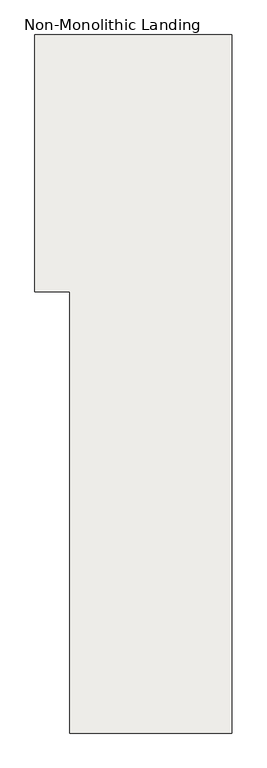
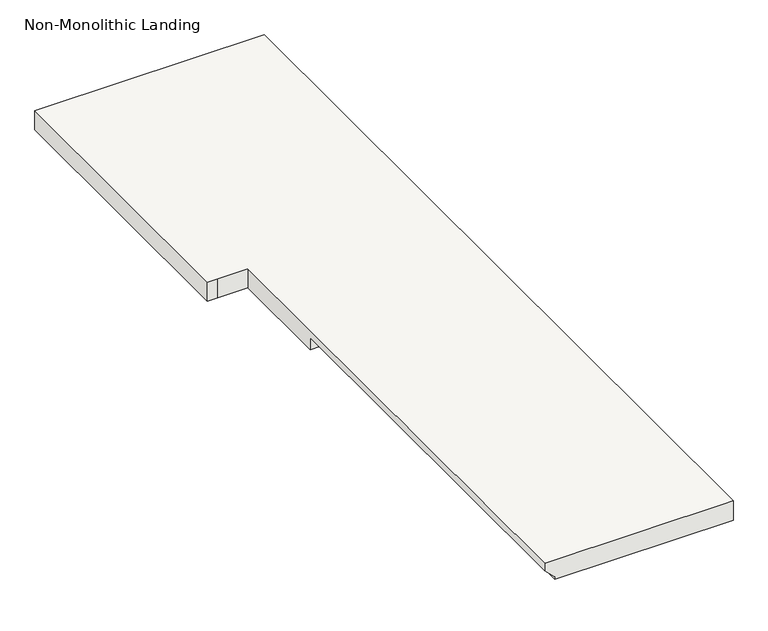
"""IFC4 building model written with IfcOpenShell, lengths in millimetres: slab geometry, Non-Monolithic Landing."""

from ifc_helpers import new_model, si_unit, origin, place, context, project, spatial, faceted_brep, source, transform, mapped, element, save


def non_monolithic_landing_8c39f4e9(model_context):
    return source(origin(), model_context, "Body", "Brep", [
        faceted_brep([(-5999.5047162, -682.6966995, 1354.6666667), (-5999.5047162, 1348.8576368, 1354.6666667), (-6546.9655018, 1348.8576368, 1354.6666667), (-6572.3655018, 1348.8576368, 1354.6666667), (-6572.3655018, 601.995692, 1354.6666667), (-6546.9655018, 601.995692, 1354.6666667), (-6470.7655018, 601.995692, 1354.6666667), (-6470.7655018, -682.6966995, 1354.6666667), (-6445.3655018, 332.8576368, 1303.8666667), (-6470.7655018, 332.8576368, 1303.8666667), (-6470.7655018, 601.995692, 1303.8666667), (-6546.9655018, 601.995692, 1303.8666667), (-6572.3655018, 601.995692, 1303.8666667), (-6572.3655018, 1348.8576368, 1303.8666667), (-6546.9655018, 1348.8576368, 1303.8666667), (-5999.5047162, 1348.8576368, 1303.8666667), (-5999.5047162, -682.6966995, 1303.8666667), (-6445.3655018, -682.6966995, 1303.8666667), (-6470.7655018, 332.8576368, 1335.6166667), (-6470.7655018, -682.6966995, 1335.6166667), (-6445.3655018, -682.6966995, 1310.2166667), (-6445.3655018, 332.8576368, 1310.2166667)], [[[0, 1, 2, 3, 4, 5, 6, 7]], [[8, 9, 10, 11, 12, 13, 14, 15, 16, 17]], [[1, 0, 16, 15]], [[3, 2, 14, 13]], [[6, 5, 11, 10]], [[7, 6, 10, 9, 18, 19]], [[2, 1, 15, 14]], [[4, 3, 13, 12]], [[20, 19, 18, 21]], [[9, 8, 21, 18]], [[8, 17, 20, 21]], [[0, 7, 19, 20, 17, 16]], [[5, 4, 12, 11]]]),
    ])


if __name__ == "__main__":
    model = new_model("IFC4")
    model_context = context("Model", 3, world=origin())
    ifc_project = project(units=[si_unit("LENGTHUNIT", "METRE", prefix="MILLI")], contexts=[model_context])
    site = spatial("IfcSite", under=ifc_project)
    building = spatial("IfcBuilding", under=site)
    placement = place(None, origin())
    non_monolithic_landing_shape = non_monolithic_landing_8c39f4e9(model_context)
    element("IfcSlab", 1, ObjectType="Non-Monolithic Landing", at=placement, inside=building, context=model_context, shape_type="MappedRepresentation", body=[
        mapped(non_monolithic_landing_shape, transform((0.0, 0.0, 0.0), x_axis=(1.0, 0.0, 0.0), y_axis=(0.0, 1.0, 0.0), z_axis=(0.0, 0.0, 1.0))),
    ])
    save(model, "model.ifc")
